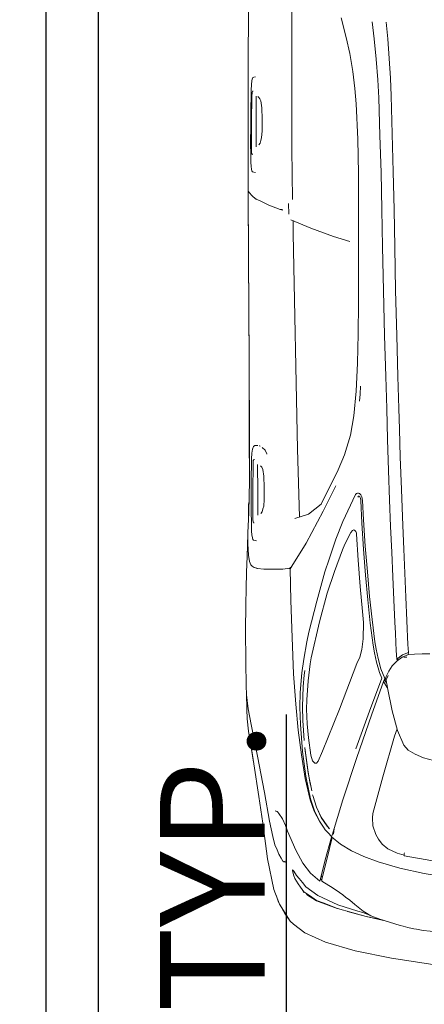
# Model space of a CAD drawing. Units: millimetres. Extents: x 595116 to 630915, y 909473 to 920225.
# Tile 5 of 134: x 629314 to 629349, y 919194 to 919279. Entities that reach past the tile are written whole.
import ezdxf

# ---------------------------------------------------------------- set-up
doc = ezdxf.new("R2010")
doc.units = ezdxf.units.MM
doc.linetypes.add('ACAD_ISO02W100', pattern=[15, 12, -3])
for name, color, linetype, lineweight in [('C-PRKG-VEHI', 8, 'Continuous', 13), ('C-PROP', 7, 'Continuous', 25), ('C-PROP-REF', 240, 'ACAD_ISO02W100', 13), ('Dimension', 3, 'Continuous', 18)]:
    doc.layers.add(name, color=color, linetype=linetype, lineweight=lineweight)
doc.styles.get("Standard").update_dxf_attribs({"font": 'arial.ttf'})
doc.dimstyles.new('ISO-25', dxfattribs={"dimtxt": 9, "dimasz": 6, "dimexe": 1.25, "dimexo": 0.625, "dimtad": 1, "dimlunit": 4, "dimtxsty": 'Standard', "dimcen": 2.5, "dimadec": 0, "dimazin": 0, "dimtfac": 1, "dimtmove": 0, "dimatfit": 3, "dimfxl": 1, "dimarcsym": 0})

# ---------------------------------------------------------------- blocks, each defined once
blk = doc.blocks.new('A$C7ADB3080')
for p, q in [((4195.1, 515.6), (4221.8, 668.4)), ((4251.7, 635.4), (4240.7, 567.6)), ((3942.5, 565.4), (3953.3, 603.8)), ((4390.5, 600.8), (4386.9, 565.1)), ((4458.5, 482.9), (4474.9, 589.7)), ((3675.1, 581.7), (3675.4, 562.4)), ((3675.4, 562.4), (3675.9, 542.6)), ((3933.6, 543.9), (3942.5, 565.4)), ((4240.7, 567.6), (4227, 505)), ((4386.9, 565.1), (4383.8, 547.2)), ((3675.9, 542.6), (3676.4, 526.7)), ((3922.9, 526.5), (3933.6, 543.9)), ((4379.1, 525.1), (4381.9, 536.1)), ((4381.9, 536.1), (4382.9, 541.1)), ((4382.9, 541.1), (4383.8, 547.2)), ((3252, 509), (3168.2, 506)), ((3168.2, 506), (3252, 509)), ((3344.7, 512.5), (3252, 509)), ((3252, 509), (3344.7, 512.5)), ((3405.5, 514.9), (3344.7, 512.5)), ((3344.7, 512.5), (3405.5, 514.9)), ((3467.2, 517.5), (3405.5, 514.9)), ((3405.5, 514.9), (3467.2, 517.5)), ((3528.9, 520.1), (3467.2, 517.5)), ((3467.2, 517.5), (3528.9, 520.1)), ((3589.5, 522.8), (3528.9, 520.1)), ((3528.9, 520.1), (3589.5, 522.8)), ((3610.4, 523.8), (3589.5, 522.8)), ((3589.5, 522.8), (3610.4, 523.8)), ((3631.1, 524.7), (3610.4, 523.8)), ((3610.4, 523.8), (3631.1, 524.7)), ((3651.3, 525.7), (3631.1, 524.7)), ((3631.1, 524.7), (3651.3, 525.7)), ((3671.3, 526.7), (3651.3, 525.7)), ((3651.3, 525.7), (3671.3, 526.7)), ((3677.3, 511.8), (3671.3, 526.7)), ((3671.3, 526.7), (3676.4, 526.5)), ((3676.4, 526.7), (3683.5, 510.8)), ((3688.7, 496.6), (3677.3, 511.8)), ((3683.5, 522.6), (3683.8, 516.7)), ((3683.5, 510.8), (3692.8, 498)), ((3683.8, 516.7), (3684.4, 515.1)), ((3872.7, 499.1), (3910.3, 515.1)), ((3910.3, 515.1), (3922.9, 526.5)), ((4188.8, 516.1), (4187.1, 516.4)), ((4193.4, 515.7), (4188.1, 497.7)), ((4188.1, 497.7), (4193.4, 515.7)), ((4195.1, 515.6), (4188.8, 516.1)), ((4198, 531.7), (4197.9, 531.2)), ((4197.9, 531.2), (4198, 531.7)), ((4373.8, 505.4), (4376, 513.6)), ((4376, 513.6), (4379.1, 525.1)), ((2239.7, 482.3), (2194, 480.4)), ((2194, 480.4), (2239.7, 482.3)), ((2337.4, 485.4), (2239.7, 482.3)), ((2239.7, 482.3), (2337.4, 485.4)), ((2434.6, 488), (2337.4, 485.4)), ((2337.4, 485.4), (2434.6, 488)), ((2531.7, 490.1), (2434.6, 488)), ((2434.6, 488), (2531.7, 490.1)), ((2628.6, 491.7), (2531.7, 490.1)), ((2531.7, 490.1), (2628.6, 491.7)), ((2740.5, 493.9), (2628.6, 491.7)), ((2628.6, 491.7), (2740.5, 493.9)), ((2856, 496.9), (2740.5, 493.9)), ((2740.5, 493.9), (2856, 496.9)), ((2961.6, 500), (2856, 496.9)), ((2856, 496.9), (2961.6, 500)), ((3043.5, 502.2), (2961.6, 500)), ((2961.6, 500), (3043.5, 502.2)), ((3097.4, 503.7), (3043.5, 502.2)), ((3043.5, 502.2), (3097.4, 503.7)), ((3168.2, 506), (3097.4, 503.7)), ((3097.4, 503.7), (3168.2, 506)), ((3347.7, 480.8), (3413.9, 483.8)), ((3413.9, 483.8), (3347.7, 480.8)), ((3413.9, 483.8), (3476.6, 486.7)), ((3476.6, 486.7), (3413.9, 483.8)), ((3476.6, 486.7), (3536.4, 489.3)), ((3536.4, 489.3), (3476.6, 486.7)), ((3536.4, 489.3), (3593.8, 491.8)), ((3593.8, 491.8), (3536.4, 489.3)), ((3593.8, 491.8), (3622.3, 493.2)), ((3622.3, 493.2), (3593.8, 491.8)), ((3622.3, 493.2), (3645.7, 494.4)), ((3645.7, 494.4), (3622.3, 493.2)), ((3645.7, 494.4), (3666.9, 495.6)), ((3666.9, 495.6), (3645.7, 494.4)), ((3666.9, 495.6), (3688.7, 496.6)), ((3688.7, 496.6), (3666.9, 495.6)), ((3687.2, 498.6), (3688.7, 498.7)), ((3691.7, 499.6), (3688.7, 496.6)), ((3688.7, 498.7), (3689.8, 497.7)), ((3692.8, 498), (3706.1, 485.3)), ((3706.1, 485.3), (3719.7, 476.4)), ((3762.8, 473.1), (3821.6, 484.9)), ((3821.6, 484.9), (3872.7, 499.1)), ((3887, 491.2), (3868.3, 497.9)), ((3868.3, 497.9), (3887, 491.2)), ((3991.5, 461.4), (3887, 491.2)), ((3887, 491.2), (3991.5, 461.4)), ((4188.1, 497.7), (4176.6, 474.1)), ((4176.6, 474.1), (4188.1, 497.7)), ((4227, 505), (4210.5, 448.6)), ((4365.6, 477.9), (4373.8, 505.4)), ((4458.5, 482.9), (4439, 389.6)), ((2093, 474.1), (2049.5, 469.8)), ((2049.5, 469.8), (2093, 474.1)), ((2143.5, 477.7), (2093, 474.1)), ((2093, 474.1), (2143.5, 477.7)), ((2194, 480.4), (2143.5, 477.7)), ((2143.5, 477.7), (2194, 480.4)), ((2341, 453.7), (2436.5, 456.4)), ((2436.5, 456.4), (2341, 453.7)), ((2436.5, 456.4), (2531.6, 458.6)), ((2531.6, 458.6), (2436.5, 456.4)), ((2531.6, 458.6), (2627.7, 460.2)), ((2627.7, 460.2), (2531.6, 458.6)), ((2627.7, 460.2), (2739.8, 462.4)), ((2739.8, 462.4), (2627.7, 460.2)), ((2739.8, 462.4), (2855.6, 465.5)), ((2855.6, 465.5), (2739.8, 462.4)), ((2855.6, 465.5), (2961.5, 468.6)), ((2961.5, 468.6), (2855.6, 465.5)), ((2961.5, 468.6), (3043.6, 470.9)), ((3043.6, 470.9), (2961.5, 468.6)), ((3043.6, 470.9), (3123.9, 472.9)), ((3123.9, 472.9), (3043.6, 470.9)), ((3123.9, 472.9), (3203.4, 475.3)), ((3203.4, 475.3), (3123.9, 472.9)), ((3203.4, 475.3), (3279, 478)), ((3279, 478), (3203.4, 475.3)), ((3279, 478), (3347.7, 480.8)), ((3347.7, 480.8), (3279, 478)), ((3713.6, 456.1), (3687.1, 448.9)), ((3687.1, 448.9), (3713.6, 456.1)), ((3713.6, 456.1), (3738.7, 466)), ((3728.7, 462.1), (3713.6, 456.1)), ((3719.7, 476.4), (3733.7, 469.8)), ((3723.1, 452.6), (3738.1, 458.5)), ((3738.7, 466), (3728.7, 462.1)), ((3730.6, 474.5), (3730.8, 474.4)), ((3730.8, 474.4), (3741.7, 469.3)), ((3733.7, 469.8), (3743.8, 466)), ((3738.1, 458.5), (3822.4, 426.8)), ((3739.1, 467.8), (3738.5, 466.1)), ((3738.5, 466.1), (3746.3, 462.9)), ((3738.7, 466.5), (3738.7, 467.9)), ((3739.5, 465.7), (3738.7, 466)), ((3738.7, 466), (3738.7, 466)), ((3741.7, 469.3), (3748.7, 470.5)), ((3743.8, 466), (3749.9, 470.8)), ((3762, 472.5), (3746.3, 462.9)), ((3832.9, 431.9), (3746.7, 463.1)), ((3748.7, 470.5), (3755.7, 471.8)), ((3755.7, 471.8), (3762.8, 473.1)), ((3762.7, 473.1), (3762, 472.5)), ((4085.9, 435.4), (3991.5, 461.4)), ((3991.5, 461.4), (4085.9, 435.4)), ((4165, 459.6), (4152.4, 450)), ((4152.4, 450), (4165, 459.6)), ((4176.6, 474.1), (4165, 459.6)), ((4165, 459.6), (4176.6, 474.1)), ((4359.8, 459.6), (4350.6, 418.1)), ((4350.6, 418.1), (4359.8, 459.6)), ((4351.4, 418), (4362.3, 467.4)), ((4357.7, 453.1), (4365.6, 477.9)), ((2048.5, 433.4), (2092.8, 438.4)), ((2092.8, 438.4), (2048.5, 433.4)), ((2092.8, 438.4), (2145.3, 443.6)), ((2145.3, 443.6), (2092.8, 438.4)), ((2145.3, 443.6), (2197.8, 447.9)), ((2197.8, 447.9), (2145.3, 443.6)), ((2197.8, 447.9), (2244.2, 450.5)), ((2244.2, 450.5), (2197.8, 447.9)), ((2244.2, 450.5), (2341, 453.7)), ((2341, 453.7), (2244.2, 450.5)), ((3587, 433.2), (3527.2, 426.8)), ((3527.2, 426.8), (3587, 433.2)), ((3643.8, 440.8), (3587, 433.2)), ((3587, 433.2), (3643.8, 440.8)), ((3596.5, 428.6), (3653.1, 436.5)), ((3662.7, 443.9), (3643.8, 440.8)), ((3643.8, 440.8), (3662.7, 443.9)), ((3653.1, 436.5), (3672.4, 439.7)), ((3687.1, 448.9), (3662.7, 443.9)), ((3662.7, 443.9), (3687.1, 448.9)), ((3672.4, 439.7), (3696.9, 445)), ((3696.9, 445), (3723.1, 452.6)), ((3941.5, 394), (3832.9, 431.9)), ((4096.8, 434.1), (4085.9, 435.4)), ((4085.9, 435.4), (4096.8, 434.1)), ((4117.8, 435.1), (4096.8, 434.1)), ((4096.8, 434.1), (4117.8, 435.1)), ((4140.4, 443), (4117.8, 435.1)), ((4117.8, 435.1), (4140.4, 443)), ((4152.4, 450), (4140.4, 443)), ((4140.4, 443), (4152.4, 450)), ((4210.5, 448.6), (4196.9, 412.4)), ((4348.9, 430.5), (4357.7, 453.1)), ((3271, 407), (3265.7, 404.2)), ((3265.7, 404.2), (3271, 407)), ((3280.2, 408.6), (3271, 407)), ((3271, 407), (3280.2, 408.6)), ((3330.4, 411.2), (3280.2, 408.6)), ((3280.2, 408.6), (3330.4, 411.2)), ((3280.2, 404.2), (3338.5, 407.1)), ((3397.7, 415.9), (3330.4, 411.2)), ((3330.4, 411.2), (3397.7, 415.9)), ((3338.5, 407.1), (3405.7, 411.7)), ((3464.1, 421.2), (3397.7, 415.9)), ((3397.7, 415.9), (3464.1, 421.2)), ((3405.7, 411.7), (3472.6, 416.8)), ((3527.2, 426.8), (3464.1, 421.2)), ((3464.1, 421.2), (3527.2, 426.8)), ((3472.6, 416.8), (3536, 422.4)), ((3501.9, 402.7), (3566, 408.5)), ((3566, 408.5), (3501.9, 402.7)), ((3536, 422.4), (3596.5, 428.6)), ((3566, 408.5), (3594.2, 410.9)), ((3594.2, 410.9), (3566, 408.5)), ((3594.2, 410.9), (3636.8, 410.4)), ((3636.8, 410.4), (3594.2, 410.9)), ((3636.8, 410.4), (3664.1, 407.1)), ((3664.1, 407.1), (3636.8, 410.4)), ((3664.1, 407.1), (3683.7, 401.7)), ((3683.7, 401.7), (3664.1, 407.1)), ((3822.4, 426.8), (3919.4, 391.3)), ((4196.9, 412.4), (4181.7, 380.2)), ((4319.8, 388.8), (4337.2, 410.2)), ((4350.6, 418.1), (4330, 344.4)), ((4330, 344.4), (4350.6, 418.1)), ((4337.1, 396.9), (4341.1, 409.4)), ((4341.1, 409.4), (4337.1, 396.9)), ((4337.2, 410.2), (4342.8, 419)), ((4338.2, 370.6), (4351.4, 418)), ((4341.1, 409.4), (4344.1, 418.1)), ((4344.1, 418.1), (4341.1, 409.4)), ((4342.8, 419), (4348.9, 430.5)), ((4344.1, 418.1), (4345.7, 423.6)), ((4345.7, 423.6), (4344.1, 418.1)), ((4345.7, 423.6), (4346.6, 426.1)), ((4346.6, 426.1), (4345.7, 423.6)), ((2130.1, 376.2), (2176.5, 383.8)), ((2176.5, 383.8), (2220.1, 389.2)), ((2220.1, 389.2), (2260.3, 392.6)), ((2260.3, 392.6), (2350.4, 396.7)), ((2350.4, 396.7), (2439.2, 398.4)), ((2439.2, 398.4), (2529.7, 398.5)), ((2529.7, 398.5), (2589.2, 398.2)), ((2589.2, 398.2), (2589.2, 398.3)), ((2618.6, 398.1), (2589.2, 398.2)), ((2618.6, 398.1), (2622.6, 398.1)), ((2622.6, 398.1), (2773, 398.1)), ((2773, 398.1), (2851.6, 397.7)), ((2851.6, 397.7), (2926.8, 396)), ((2926.8, 396), (2999.6, 392.2)), ((2986.1, 403.8), (3006.7, 402.9)), ((2999.6, 392.2), (3062.7, 386.1)), ((3006.7, 402.9), (3025.1, 400.8)), ((3062.7, 386.1), (3112.6, 377.8)), ((3262.3, 400.8), (3261.6, 398.5)), ((3261.6, 398.5), (3262.3, 400.8)), ((3261.6, 398.5), (3261.6, 396.3)), ((3261.6, 396.3), (3261.6, 398.5)), ((3261.6, 396.4), (3261.6, 396.3)), ((3261.6, 396.3), (3262.5, 393.6)), ((3262.5, 393.6), (3261.6, 396.3)), ((3262.3, 400.8), (3262.2, 400.6)), ((3265.7, 404.2), (3262.3, 400.8)), ((3262.3, 400.8), (3265.7, 404.2)), ((3262.5, 393.6), (3264.7, 391.1)), ((3264.7, 391.1), (3262.5, 393.6)), ((3264.7, 391.1), (3334.6, 357.8)), ((3334.6, 357.8), (3264.7, 391.1)), ((3269.2, 399.3), (3271, 401.5)), ((3269.6, 398.5), (3269.5, 399.6)), ((3271.9, 397.1), (3269.6, 398.5)), ((3271, 401.5), (3274.3, 403.3)), ((3274.3, 403.3), (3280.2, 404.2)), ((3356.4, 386.7), (3357.6, 389.2)), ((3357.6, 389.2), (3356.4, 386.7)), ((3357.5, 383.2), (3356.4, 386.7)), ((3356.4, 386.7), (3357.5, 383.2)), ((3363.1, 378.6), (3357.5, 383.2)), ((3357.5, 383.2), (3363.1, 378.6)), ((3357.6, 389.2), (3360.3, 391.7)), ((3360.3, 391.7), (3357.6, 389.2)), ((3360.3, 391.7), (3364.2, 393)), ((3364.2, 393), (3360.3, 391.7)), ((3361.1, 391.9), (3360.3, 391.7)), ((3364.2, 393), (3366.9, 393.4)), ((3366.9, 393.4), (3364.2, 393)), ((3366.9, 393.4), (3366.5, 393.3)), ((3366.9, 393.4), (3434.5, 397.6)), ((3434.5, 397.6), (3366.9, 393.4)), ((3434.5, 397.6), (3501.9, 402.7)), ((3501.9, 402.7), (3434.5, 397.6)), ((3683.7, 401.7), (3700.4, 394)), ((3700.4, 394), (3683.7, 401.7)), ((3700.4, 394), (3817.2, 349.4)), ((3817.2, 349.4), (3700.4, 394)), ((4050.4, 358), (3941.5, 394)), ((4181.7, 380.2), (4164.8, 352.2)), ((4309, 375.9), (4319.8, 388.8)), ((4321.2, 345.1), (4337.1, 396.9)), ((4337.1, 396.9), (4321.2, 345.1)), ((4439, 389.6), (4416.8, 313.9)), ((2038.3, 354.2), (2088.8, 367)), ((2088.8, 367), (2130.1, 376.2)), ((2601.1, 334.3), (2614.2, 376.3)), ((3112.6, 377.8), (3163.1, 362.7)), ((3163.1, 362.7), (3201.4, 346.4)), ((3334.6, 357.8), (3380.1, 340.6)), ((3380.1, 340.6), (3334.6, 357.8)), ((3392.8, 363.5), (3363.1, 378.6)), ((3363.1, 378.6), (3392.8, 363.5)), ((3407.4, 357), (3392.8, 363.5)), ((3392.8, 363.5), (3407.4, 357)), ((3463.6, 336.8), (3407.4, 357)), ((3407.4, 357), (3463.6, 336.8)), ((4142, 330.4), (4050.4, 358)), ((4289.5, 349.4), (4295.4, 357.9)), ((4295.4, 357.9), (4301.5, 365.2)), ((4301.5, 365.2), (4309, 375.9)), ((2579.5, 276.2), (2601.1, 334.3)), ((3201.4, 346.4), (3289.8, 302.1)), ((3242.7, 339.9), (3307.9, 307.6)), ((3380.1, 340.6), (3431.3, 322.8)), ((3431.3, 322.8), (3380.1, 340.6)), ((3519.3, 317.6), (3463.6, 336.8)), ((3463.6, 336.8), (3519.3, 317.6)), ((3817.2, 349.4), (3925.2, 306)), ((3925.2, 306), (3817.2, 349.4)), ((4125, 335.6), (4138.5, 334.1)), ((4137.7, 333.1), (4138.9, 334.6)), ((4137.7, 333.1), (4139.4, 331.5)), ((4139.4, 331.5), (4146.3, 328.7)), ((4140.7, 330.9), (4140.8, 330.9)), ((4164.8, 352.2), (4146.3, 328.7)), ((4147.7, 330.5), (4204.1, 316.7)), ((4259.7, 303.9), (4278, 333.2)), ((4278, 333.2), (4289.5, 349.4)), ((4297.1, 293.6), (4321.2, 345.1)), ((4321.2, 345.1), (4297.1, 293.6)), ((4310.5, 290.6), (4330.7, 343.8)), ((4330, 344.4), (4316, 307.6)), ((4316, 307.6), (4330, 344.4)), ((3307.9, 307.6), (3390, 263.8)), ((3431.3, 322.8), (3463.8, 312.3)), ((3463.8, 312.3), (3431.3, 322.8)), ((3463.8, 312.3), (3540, 291.3)), ((3540, 291.3), (3463.8, 312.3)), ((3592.6, 298), (3519.3, 317.6)), ((3519.3, 317.6), (3592.6, 298)), ((3925.2, 306), (3951.6, 295.2)), ((3951.6, 295.2), (3925.2, 306)), ((4095.5, 302.7), (4117.9, 317.7)), ((4118.4, 317.6), (4096.4, 302.9)), ((4120.9, 308.2), (4106, 297.8)), ((4117.9, 317.7), (4125.2, 324.1)), ((4125.2, 323.9), (4118.4, 317.6)), ((4121.1, 308.3), (4120.9, 308.2)), ((4121.2, 308.4), (4128, 313.1)), ((4125, 323.9), (4125.2, 323.9)), ((4128, 313.1), (4136.9, 321.3)), ((4134.9, 319.4), (4134.8, 319.4)), ((4145.3, 329.1), (4134.9, 319.4)), ((4136.9, 321.3), (4145.3, 329.1)), ((4204.9, 312.9), (4146.6, 329.1)), ((4204.1, 316.7), (4248.1, 305.5)), ((4250.9, 301.7), (4204.9, 312.9)), ((4249, 305.3), (4246.7, 302.7)), ((4248.1, 305.5), (4256.1, 303.9)), ((4256.6, 304.1), (4256.3, 303.5)), ((4316, 307.6), (4309.4, 290.9)), ((4309.4, 290.9), (4316, 307.6)), ((4416.8, 313.9), (4392.6, 260.2)), ((3289.8, 302.1), (3315.3, 269.6)), ((3540, 291.3), (3619.1, 270.6)), ((3619.1, 270.6), (3540, 291.3)), ((3685.5, 277), (3592.6, 298)), ((3592.6, 298), (3685.5, 277)), ((3950.2, 280), (3936.2, 276.1)), ((3936.2, 276.1), (3950.2, 280)), ((3956.1, 285.8), (3950.2, 280)), ((3950.2, 280), (3956.1, 285.8)), ((3951.6, 295.2), (3956, 290.8)), ((3956, 290.8), (3951.6, 295.2)), ((3956, 290.8), (3956.1, 285.8)), ((3956.1, 285.8), (3956, 290.8)), ((4039.3, 280.8), (4038.1, 280.6)), ((4039.2, 280.8), (4041.7, 281.6)), ((4069.8, 290.4), (4039.3, 280.8)), ((4048.1, 275.3), (4078.8, 285.1)), ((4078.8, 285.1), (4048.1, 275.3)), ((4050.7, 274.3), (4080.1, 284.6)), ((4080.1, 284.6), (4050.7, 274.3)), ((4069.4, 290.3), (4095.5, 302.7)), ((4096.4, 302.9), (4069.8, 290.4)), ((4078.8, 285.1), (4106, 297.8)), ((4106, 297.8), (4078.8, 285.1)), ((4080.1, 284.6), (4106, 297.8)), ((4106, 297.8), (4080.1, 284.6)), ((4106, 297.8), (4109.2, 300.1)), ((4239.6, 275.2), (4260.4, 299.4)), ((4260.4, 299.4), (4250.9, 301.7)), ((4256.3, 303.5), (4254.1, 300.9)), ((4256.1, 303.9), (4256.5, 303.9)), ((4257.4, 303.9), (4259.7, 303.9)), ((4274.7, 262.9), (4297.1, 293.6)), ((4297.1, 293.6), (4274.7, 262.9)), ((4301.5, 278.7), (4290.4, 262.4)), ((4290.4, 262.4), (4301.5, 278.7)), ((4294, 264.8), (4310.5, 290.6)), ((4309.4, 290.9), (4301.5, 278.7)), ((4301.5, 278.7), (4309.4, 290.9)), ((2558, 224.3), (2579.5, 276.2)), ((3315.3, 269.6), (3327.1, 234.4)), ((3390, 263.8), (3456.6, 223)), ((3619.1, 270.6), (3644.1, 265.3)), ((3644.1, 265.3), (3619.1, 270.6)), ((3644.1, 265.3), (3689.1, 258)), ((3689.1, 258), (3644.1, 265.3)), ((3701, 274.5), (3685.5, 277)), ((3685.5, 277), (3701, 274.5)), ((3689.1, 258), (3724.3, 252.9)), ((3724.3, 252.9), (3689.1, 258)), ((3744.9, 269.5), (3701, 274.5)), ((3701, 274.5), (3744.9, 269.5)), ((3730.4, 259), (3718.4, 260.4)), ((3759.2, 256.3), (3730.4, 259)), ((3793.1, 266), (3744.9, 269.5)), ((3744.9, 269.5), (3793.1, 266)), ((3811.2, 254.5), (3759.2, 256.3)), ((3817.7, 265.2), (3793.1, 266)), ((3793.1, 266), (3817.7, 265.2)), ((3846.5, 255.3), (3811.2, 254.5)), ((3854.8, 266.4), (3817.7, 265.2)), ((3817.7, 265.2), (3854.8, 266.4)), ((3898.3, 259.2), (3846.5, 255.3)), ((3891.3, 269.6), (3854.8, 266.4)), ((3854.8, 266.4), (3891.3, 269.6)), ((3856.9, 249.1), (3926.7, 254.9)), ((3926.7, 254.9), (3856.9, 249.1)), ((3936.2, 276.1), (3891.3, 269.6)), ((3891.3, 269.6), (3936.2, 276.1)), ((3917.5, 260.6), (3916, 260.5)), ((3917.1, 260.6), (3979.7, 268.9)), ((3981.3, 269), (3917.5, 260.6)), ((3926.7, 254.9), (3990.3, 263.5)), ((3990.3, 263.5), (3926.7, 254.9)), ((3935.4, 251.6), (3995.6, 261.5)), ((3979.7, 268.9), (4004.3, 273.7)), ((4027.9, 278.5), (3981.3, 269)), ((3990.3, 263.5), (4048.1, 275.3)), ((4048.1, 275.3), (3990.3, 263.5)), ((3995.6, 261.5), (4050.7, 274.3)), ((4004.3, 273.7), (4013.3, 275.5)), ((4180, 237.5), (4213.7, 255.4)), ((4213.7, 255.4), (4239.6, 275.2)), ((4253.1, 245.9), (4263.7, 254.4)), ((4263.7, 254.4), (4253.1, 245.9)), ((4263.7, 254.4), (4274.7, 262.9)), ((4274.7, 262.9), (4263.7, 254.4)), ((4287.1, 257.7), (4275.4, 249.2)), ((4275.4, 249.2), (4287.1, 257.7)), ((4290.4, 262.4), (4287.1, 257.7)), ((4287.1, 257.7), (4290.4, 262.4)), ((4287.4, 255.8), (4288.8, 256.8)), ((4392.6, 260.2), (4370.3, 231.3)), ((2375.6, 227.4), (2506, 229.2)), ((2560.4, 230.1), (2594.2, 230.7)), ((2594.2, 230.7), (3148.3, 241.7)), ((3148.3, 241.7), (3323, 246.6)), ((3632.9, 227.7), (3726.9, 231.8)), ((3724.3, 252.9), (3774.5, 248.5)), ((3774.5, 248.5), (3724.3, 252.9)), ((3726.9, 231.8), (3804.6, 237)), ((3774.5, 248.5), (3812.3, 247.8)), ((3812.3, 247.8), (3774.5, 248.5)), ((3804.6, 237), (3871.4, 243.6)), ((3812.3, 247.8), (3856.9, 249.1)), ((3856.9, 249.1), (3812.3, 247.8)), ((3871.4, 243.6), (3935.4, 251.6)), ((4131.6, 216.2), (4180, 237.5)), ((4230.6, 228.5), (4234.6, 232)), ((4234.6, 232), (4230.6, 228.5)), ((4233.3, 228.6), (4230.6, 228.5)), ((4230.6, 228.5), (4233.3, 228.6)), ((4246.7, 232.5), (4233.3, 228.6)), ((4233.3, 228.6), (4246.7, 232.5)), ((4234.6, 232), (4245.3, 239.2)), ((4245.3, 239.2), (4234.6, 232)), ((4245.3, 239.2), (4253.1, 245.9)), ((4253.1, 245.9), (4245.3, 239.2)), ((4252.8, 234.9), (4246.7, 232.5)), ((4246.7, 232.5), (4252.8, 234.9)), ((4259.8, 238.8), (4252.8, 234.9)), ((4252.8, 234.9), (4259.8, 238.8)), ((4266.7, 243.2), (4259.8, 238.8)), ((4259.8, 238.8), (4266.7, 243.2)), ((4275.4, 249.2), (4266.7, 243.2)), ((4266.7, 243.2), (4275.4, 249.2)), ((4363.1, 223.2), (4370.3, 231.3)), ((1724.4, 226.9), (2375.6, 227.4)), ((2516.3, 218.5), (2543.4, 219)), ((2532.1, 203.2), (2532.1, 196.8)), ((3452.5, 222.4), (3455.3, 222.5)), ((3455.5, 223.2), (3452.6, 225.5)), ((3456.9, 204.1), (3454.3, 222.4)), ((3455.3, 223.3), (3455.3, 223.8)), ((3455.3, 219), (3455.3, 223.2)), ((3456.6, 223), (3537.8, 224.8)), ((3456.9, 204.1), (3456.9, 183.7)), ((3537.8, 224.8), (3632.9, 227.7)), ((4086.1, 193.8), (4099.9, 203.1)), ((4099.9, 203.1), (4116.9, 211.1)), ((4116.9, 211.1), (4131.6, 216.2)), ((4201, 199.3), (4208.9, 204)), ((4210.6, 206.2), (4208.9, 209.9)), ((4210.6, 206.2), (4208.9, 204)), ((4209.1, 209.5), (4211.3, 210.3)), ((4210.4, 207.6), (4210, 207.4)), ((4211.4, 210.7), (4210.4, 207.6)), ((4319.2, 195.6), (4363.1, 223.2)), ((4343.6, 209.1), (4323.2, 198.1)), ((4363.1, 223.2), (4343.6, 209.1)), ((2520.5, 167.9), (2532.1, 196.8)), ((2532.1, 202.6), (2533.9, 202.6)), ((2533.9, 202.6), (2534.6, 202.6)), ((3456.9, 183.7), (3456.9, 155)), ((4079.5, 184.4), (4080, 186.8)), ((4079.8, 186.2), (4081, 189)), ((4081, 189), (4082.5, 190.8)), ((4082.5, 190.8), (4086.1, 193.8)), ((4125.1, 173.9), (4145.5, 178.6)), ((4145.5, 178.6), (4166.8, 183.6)), ((4166.8, 183.6), (4179.6, 189)), ((4179.6, 189), (4190.3, 193.8)), ((4190.3, 193.8), (4201, 199.3)), ((4202.8, 164.9), (4281.2, 180.9)), ((4281.2, 180.9), (4319.2, 195.6)), ((4314.2, 193.2), (4296.1, 186.6)), ((4319.2, 195.6), (4314.2, 193.2)), ((2510.7, 147.4), (2520.5, 167.9)), ((3143.9, 150.5), (3151.3, 158.6)), ((3151.3, 158.6), (3160.5, 162.6)), ((3160.5, 162.6), (3161.6, 162.7)), ((3194.7, 149.8), (3200.5, 152.6)), ((3200.5, 152.6), (3218.3, 154.9)), ((3218.3, 154.9), (3247.2, 156.3)), ((3247.2, 156.3), (3278.4, 156)), ((3278.4, 156), (3294.9, 154.7)), ((3294.9, 154.7), (3301.9, 152.9)), ((3301.9, 152.9), (3309.3, 150.8)), ((3456.9, 155), (3455.4, 139.2)), ((3938.8, 138.5), (4032, 156.5)), ((4032, 156.5), (4106, 169.6)), ((4110.6, 152.5), (4042.4, 142.3)), ((4106, 169.6), (4125.1, 173.9)), ((4110.6, 152.5), (4202.8, 164.9)), ((2191.2, 129), (2190.4, 134.1)), ((2191.2, 129), (2193.4, 126.4)), ((2226.9, 128.1), (2227.3, 126.2)), ((2309.6, 135.8), (2240, 135.5)), ((2241.1, 139.3), (2243.3, 141.9)), ((2243.3, 141.9), (2246.7, 145.1)), ((2246.7, 145.1), (2252.5, 147.6)), ((2252.5, 147.6), (2270.3, 149.7)), ((2270.3, 149.7), (2299.3, 150.8)), ((2299.3, 150.8), (2330.4, 150.4)), ((2370.7, 135.5), (2309.6, 135.8)), ((2330.4, 150.4), (2346.9, 149.1)), ((2346.9, 149.1), (2354, 147.3)), ((2354, 147.3), (2361.4, 145.4)), ((2361.4, 145.4), (2365.7, 142)), ((2389.9, 127.1), (2389.6, 124.9)), ((2434.5, 125.7), (2435.7, 129.1)), ((2435.7, 129.1), (2436.2, 134.1)), ((2496.6, 124.8), (2503.9, 133.7)), ((2503.9, 133.7), (2504.3, 134.2)), ((2504.3, 134.2), (2505, 135.5)), ((2505, 135.5), (2510.7, 147.4)), ((3138.8, 135.8), (3139.2, 139.9)), ((3138.9, 134.8), (3138.8, 135.8)), ((3139.2, 131.8), (3138.8, 134.4)), ((3139.2, 131.8), (3141.5, 128.4)), ((3139.6, 143.6), (3140.7, 145.3)), ((3139.6, 142.8), (3139.6, 143.6)), ((3141.5, 128.4), (3148.6, 125.9)), ((3143.8, 150.4), (3143.9, 150.5)), ((3174.9, 131), (3175.3, 129)), ((3176.5, 128.4), (3175.3, 129)), ((3176.5, 128.4), (3177.6, 128.1)), ((3177.6, 128.1), (3180.9, 127.5)), ((3180.9, 127.5), (3185.7, 127.3)), ((3185.7, 127.3), (3257.4, 126.7)), ((3257.6, 139.9), (3187.9, 139.2)), ((3191.3, 146.3), (3194.7, 149.8)), ((3257.4, 126.7), (3325.3, 126.6)), ((3318.7, 139.9), (3257.6, 139.9)), ((3309.3, 150.8), (3313.6, 147.2)), ((3325.3, 126.6), (3330.2, 126.7)), ((3330.2, 126.7), (3334.3, 127.3)), ((3334.3, 127.3), (3336.4, 128.1)), ((3335.7, 127.5), (3334.5, 127.3)), ((3337.6, 128.4), (3335.7, 127.5)), ((3336.4, 128.1), (3337.6, 128.4)), ((3338, 130.6), (3337.6, 128.4)), ((3376.8, 125.6), (3380.5, 126.9)), ((3380.5, 126.9), (3382.5, 128.9)), ((3382.5, 128.9), (3383.7, 133.3)), ((3383.7, 133.3), (3384, 136.4)), ((3453.1, 130.6), (3449.9, 125.3)), ((3454.9, 136.7), (3453.1, 130.6)), ((3455.1, 137.4), (3454.9, 136.7)), ((3455.4, 139.2), (3455.1, 137.4)), ((3856.8, 122.3), (3938.8, 138.5)), ((3958, 129.3), (3891.5, 119.3)), ((3937.3, 125.8), (3954.2, 128.7)), ((4042.4, 142.3), (3958, 129.3)), ((2187.9, 115), (1717.5, 115.9)), ((2484.5, 114.5), (2187.9, 115)), ((2193.4, 126.4), (2200.6, 124.5)), ((2200.6, 124.5), (2210.5, 123.4)), ((2210.5, 123.4), (2224.9, 122.7)), ((2241, 122.3), (2224.9, 122.7)), ((2228.5, 125.6), (2227.3, 126.2)), ((2228.5, 125.6), (2229.6, 125.3)), ((2229.6, 125.3), (2232.9, 124.8)), ((2232.9, 124.8), (2237.6, 124.6)), ((2237.6, 124.6), (2309.4, 123.8)), ((2270.8, 121.8), (2241, 122.3)), ((2301.2, 121.5), (2270.8, 121.8)), ((2330.4, 121.3), (2301.2, 121.5)), ((2309.4, 123.8), (2377.2, 123.3)), ((2346.2, 121.2), (2330.4, 121.3)), ((2361.6, 121.2), (2346.2, 121.2)), ((2390.1, 121.5), (2361.6, 121.2)), ((2377.2, 123.3), (2382.2, 123.4)), ((2382.2, 123.4), (2386.2, 123.8)), ((2386.2, 123.8), (2388.4, 124.5)), ((2387.6, 124.1), (2386.9, 124)), ((2389.6, 124.9), (2387.6, 124.1)), ((2388.4, 124.5), (2389.6, 124.9)), ((2390.1, 121.5), (2411.1, 121.9)), ((2411.1, 121.9), (2420.6, 122.4)), ((2420.6, 122.4), (2428.8, 123.3)), ((2428.8, 123.3), (2432.5, 124.2)), ((2432.5, 124.2), (2434.5, 125.7)), ((2484.5, 114.5), (2494.5, 123.1)), ((2485.3, 114.8), (2484.9, 114.8)), ((2485.3, 114.8), (2485.1, 115)), ((2485.4, 114.8), (2485.3, 114.8)), ((2485.4, 114.8), (2654.1, 115.7)), ((2494.5, 123.1), (2496.6, 124.8)), ((2652.6, 115.6), (2496.9, 114.9)), ((2920.1, 117), (2652.6, 115.6)), ((2924.7, 117.2), (2654.1, 115.7)), ((2920.1, 117), (3154.5, 117.7)), ((3118.4, 117.9), (2924.7, 117.2)), ((2925, 117.2), (3141.2, 118)), ((2925.4, 117.2), (2925, 117.2)), ((3141.2, 118), (3155.1, 118)), ((3148.6, 125.9), (3158.6, 124.6)), ((3189.7, 117.9), (3154.5, 117.7)), ((3167.2, 118), (3155.1, 118)), ((3155.1, 118), (3167.6, 118)), ((3167.2, 118), (3155.1, 118)), ((3158.6, 124.6), (3173, 123.7)), ((3179.8, 118), (3167.2, 118)), ((3167.2, 118), (3167.6, 118)), ((3189, 123.3), (3173, 123.7)), ((3189.8, 117.9), (3179.8, 118)), ((3218.8, 122.8), (3189, 123.3)), ((3230.4, 117.9), (3189.7, 117.9)), ((3249.2, 122.6), (3218.8, 122.8)), ((3230.4, 117.9), (3269.2, 117.1)), ((3278.5, 122.4), (3249.2, 122.6)), ((3269.2, 117.1), (3311.5, 116.3)), ((3294.3, 122.5), (3278.5, 122.4)), ((3285.8, 116.8), (3290.9, 115.9)), ((3290.9, 115.9), (3301, 115.9)), ((3309.6, 122.6), (3294.3, 122.5)), ((3301, 115.9), (3322.7, 115.9)), ((3338.2, 123), (3309.6, 122.6)), ((3311.5, 116.3), (3363.4, 114.4)), ((3338.2, 123), (3359.1, 123.7)), ((3359.1, 123.7), (3368.6, 124.4)), ((3363.4, 114.4), (3392, 114.3)), ((3366.1, 114.4), (3424.7, 112.1)), ((3368.6, 124.4), (3376.8, 125.6)), ((3392, 114.3), (3420.9, 115.7)), ((3420.9, 115.7), (3437.5, 118)), ((3424.7, 112.1), (3465.3, 110.6)), ((3437.5, 118), (3445.8, 121.5)), ((3449.9, 125.3), (3445.8, 121.5)), ((3465.3, 110.6), (3506.8, 109.4)), ((3506.8, 109.4), (3548.4, 108.5)), ((3548.4, 108.5), (3615.8, 107.9)), ((3615.8, 107.9), (3693.3, 108.5)), ((3693.3, 108.5), (3760.4, 109.8)), ((3777.5, 110.4), (3760.4, 109.8)), ((3777.5, 110.4), (3780.6, 110.6)), ((3817, 111.7), (3777.6, 110.4)), ((3777.6, 110.4), (3817.8, 111.5)), ((3780.6, 110.6), (3816.5, 114.7)), ((3816.5, 114.7), (3856.8, 122.3)), ((3817.8, 111.5), (3842, 112.3)), ((3842, 112.3), (3873.8, 116)), ((3937.3, 125.8), (3873.8, 116))]:
    blk.add_line(p, q)
blk = doc.blocks.new('*D155')
at = {"layer": 'Defpoints', "color": 0, "transparency": 16777216}
for p in [(629334.041, 919150.928), (629336.741, 919150.928), (629334.041, 919141.928)]:
    blk.add_point(p, dxfattribs=at)
at = {"layer": 'Dimension', "color": 0, "lineweight": -2, "transparency": 16777216}
for p, q in [((629336.741, 919156.928), (629336.741, 919219.037)), ((629334.666, 919150.928), (629337.991, 919150.928)), ((629336.741, 919141.928), (629336.741, 919150.928)), ((629334.666, 919141.928), (629337.991, 919141.928)), ((629336.741, 919135.928), (629336.741, 919129.928))]:
    blk.add_line(p, q, dxfattribs=at)
at = {"layer": 'Dimension', "color": 0, "transparency": 16777216}
for points in [[(629335.741, 919156.928), (629337.741, 919156.928), (629336.741, 919150.928)], [(629335.741, 919135.928), (629337.741, 919135.928), (629336.741, 919141.928)]]:
    blk.add_solid(points, dxfattribs=at)
at = {"layer": 'Dimension', "color": 0, "transparency": 16777216, "insert": (629331.521, 919190.982), "char_height": 9, "attachment_point": 5, "rotation": 90}
blk.add_mtext('0\'-9" TYP.', dxfattribs=at)
blk = doc.blocks.new('*D215')
at = {"layer": 'Defpoints', "color": 0, "transparency": 16777216}
for p in [(629316.041, 919411.828), (629505.041, 919411.828), (629505.041, 918832.378)]:
    blk.add_point(p, dxfattribs=at)
at = {"layer": 'Dimension', "color": 0, "lineweight": -2, "transparency": 16777216}
for p, q in [((629316.041, 919411.203), (629316.041, 918831.128)), ((629505.041, 919411.203), (629505.041, 918831.128)), ((629322.041, 918832.378), (629499.041, 918832.378))]:
    blk.add_line(p, q, dxfattribs=at)
at = {"layer": 'Dimension', "color": 0, "transparency": 16777216}
for points in [[(629322.041, 918833.378), (629322.041, 918831.378), (629316.041, 918832.378)], [(629499.041, 918833.378), (629499.041, 918831.378), (629505.041, 918832.378)]]:
    blk.add_solid(points, dxfattribs=at)
at = {"layer": 'Dimension', "color": 0, "transparency": 16777216, "insert": (629410.541, 918837.598), "char_height": 9, "attachment_point": 5}
blk.add_mtext('15\'-9"', dxfattribs=at)
blk = doc.blocks.new('*D221')
at = {"layer": 'Defpoints', "color": 0, "transparency": 16777216}
for p in [(629511.274, 919302.009), (629155.382, 919160.917), (629511.274, 919160.917)]:
    blk.add_point(p, dxfattribs=at)
at = {"layer": 'Dimension', "color": 0, "lineweight": -2, "transparency": 16777216}
for p, q in [((629510.649, 919302.009), (629154.132, 919302.009)), ((629155.382, 919296.009), (629155.382, 919166.917)), ((629510.649, 919160.917), (629154.132, 919160.917))]:
    blk.add_line(p, q, dxfattribs=at)
at = {"layer": 'Dimension', "color": 0, "transparency": 16777216}
for points in [[(629154.382, 919296.009), (629156.382, 919296.009), (629155.382, 919302.009)], [(629154.382, 919166.917), (629156.382, 919166.917), (629155.382, 919160.917)]]:
    blk.add_solid(points, dxfattribs=at)
at = {"layer": 'Dimension', "color": 0, "transparency": 16777216, "insert": (629150.162, 919231.463), "char_height": 9, "attachment_point": 5, "rotation": 90}
blk.add_mtext('11\'-9"', dxfattribs=at)

msp = doc.modelspace()

# ---------------------------------------------------------------- linework, layer by layer
at = {"layer": 'C-PROP'}
msp.add_line((629320.541, 919345.928), (629320.541, 919150.928), dxfattribs=at)
at = {"layer": 'C-PROP-REF'}
msp.add_line((629316.041, 919146.428), (629316.041, 920084.928), dxfattribs=at)

# ---------------------------------------------------------------- block references
at = {"layer": 'C-PRKG-VEHI', "xscale": 0.0334614614063694, "yscale": 0.0334614614063694, "zscale": 0.0334614614063694, "rotation": 270}
msp.add_blockref('A$C7ADB3080', (629329.6, 919347.236), dxfattribs=at)

# ---------------------------------------------------------------- dimensions: what is measured, and where the dimension line sits
at = {"layer": 'Dimension'}
dim = msp.add_linear_dim(base=(629505.041, 918832.378), p1=(629316.041, 919411.828), p2=(629505.041, 919411.828), dimstyle='ISO-25', override={"dimdec": 1, "dimlfac": 1, "dimrnd": 0, "dimzin": 1, "dimdsep": 46, "dimlunit": 4, "dimfrac": 2}, dxfattribs=at)
dim.commit()
dim.dimension.update_dxf_attribs({"geometry": '*D215', "text_midpoint": (629410.541, 918837.598)})
dim = msp.add_linear_dim(base=(629155.382, 919160.917), p1=(629511.274, 919302.009), p2=(629511.274, 919160.917), angle=90, dimstyle='ISO-25', override={"dimdec": 1, "dimlfac": 1, "dimrnd": 0, "dimzin": 1, "dimdsep": 46, "dimlunit": 4, "dimfrac": 2}, dxfattribs=at)
dim.commit()
dim.dimension.update_dxf_attribs({"geometry": '*D221', "text_midpoint": (629150.162, 919231.463)})
dim = msp.add_linear_dim(base=(629336.741, 919150.928), p1=(629334.041, 919141.928), p2=(629334.041, 919150.928), angle=90, text='<> TYP.', dimstyle='ISO-25', override={"dimdec": 1, "dimlfac": 1, "dimrnd": 0, "dimzin": 1, "dimdsep": 46, "dimlunit": 4, "dimfrac": 2}, dxfattribs=at)
dim.commit()
dim.dimension.update_dxf_attribs({"geometry": '*D155', "text_midpoint": (629331.521, 919190.982)})

doc.saveas('drawing.dxf')
